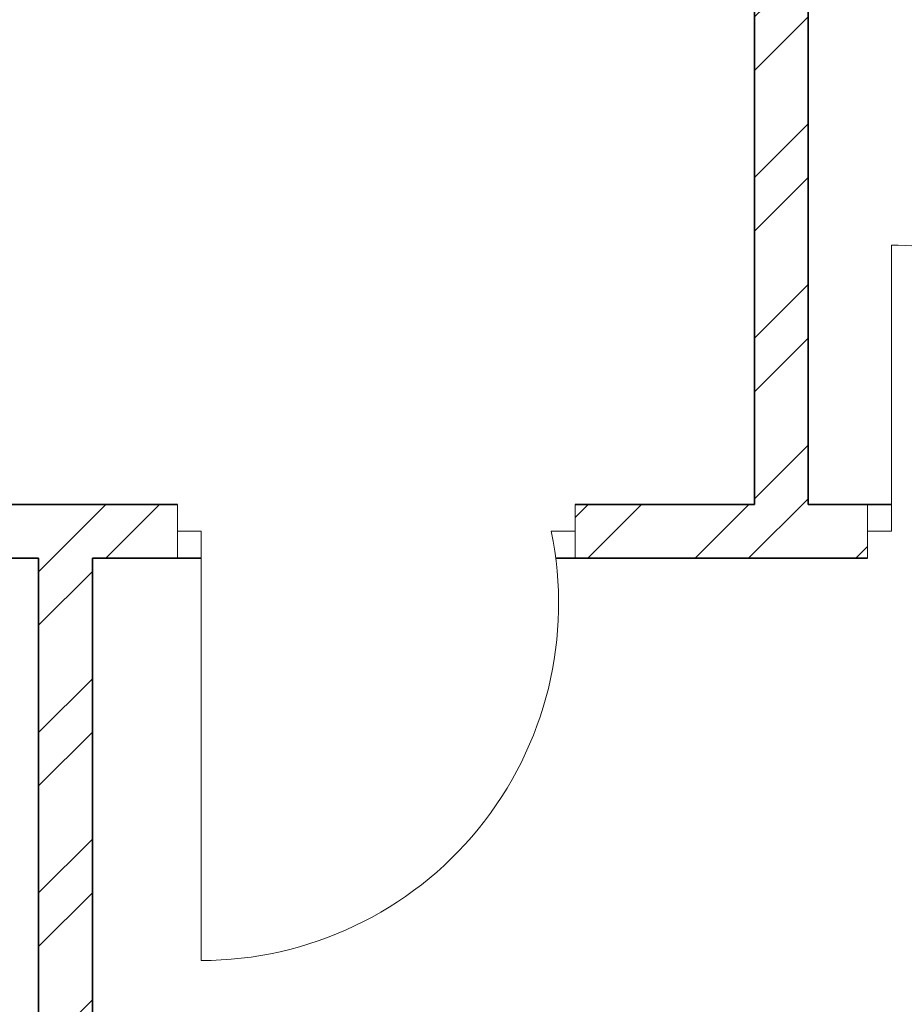
# Model space of a CAD drawing. Units: inches. Extents: x 1962 to 2771, y 1245 to 2660.
# Tile 14 of 114: x 2506 to 2580, y 1609 to 1692. Entities that reach past the tile are written whole.
import ezdxf

# ---------------------------------------------------------------- set-up
doc = ezdxf.new("R2010")
doc.units = ezdxf.units.IN
for name, color, linetype, lineweight in [('A-DOOR', 3, 'Continuous', 18), ('A-WALL', 7, 'Continuous', 35), ('A-WALL-PATT', 252, 'Continuous', 13)]:
    doc.layers.add(name, color=color, linetype=linetype, lineweight=lineweight)

msp = doc.modelspace()

# ---------------------------------------------------------------- hatches: boundary and pattern name
at = {"layer": 'A-WALL-PATT'}
h = msp.add_hatch(dxfattribs=at)
h.set_pattern_fill('ANSI32', color=256)
h.paths.add_polyline_path([(2090.8074, 2467.3437), (2141.6481, 2467.3437), (2141.6481, 2469.5937), (2141.6481, 2471.8437), (2086.3074, 2471.8437), (2086.3074, 2422.5333), (2090.8074, 2422.5333)])
h.paths.add_polyline_path([(2282.7664, 2471.8437), (2204.8982, 2471.8437), (2204.8982, 2467.3437), (2234.8074, 2467.3437), (2234.8074, 2311.3437), (2228.7492, 2311.3437), (2228.7492, 2306.8437), (2234.8074, 2306.8437), (2331.9227, 2306.8437), (2331.9227, 2309.0937), (2331.9227, 2311.3437), (2239.3074, 2311.3437), (2239.3074, 2467.3437), (2282.7664, 2467.3437), (2282.7664, 2469.5937)])
h.paths.add_polyline_path([(2471.4531, 2519.8437), (2552.011, 2519.8437), (2564.3996, 2519.8437), (2564.3996, 2511.1389), (2568.8996, 2511.1389), (2568.8996, 2524.3437), (2466.9531, 2524.3437), (2466.9531, 2471.8437), (2450.0749, 2471.8437), (2446.4672, 2471.8437), (2446.4672, 2467.3437), (2450.0749, 2467.3437), (2475.9988, 2467.3437), (2475.9988, 2469.5937), (2475.9988, 2471.8437), (2471.4531, 2471.8437)])
h.paths.add_polyline_path([(2575.2231, 2469.5937), (2575.2231, 2471.8437), (2568.8996, 2471.8437), (2568.8996, 2487.1389), (2564.3996, 2487.1389), (2564.3996, 2471.8437), (2556.511, 2471.8437), (2499.2904, 2471.8437), (2499.2904, 2467.3437), (2507.8074, 2467.3437), (2507.8074, 2311.3437), (2414.863, 2311.3437), (2414.863, 2306.8437), (2512.3074, 2306.8437), (2517.0114, 2306.8437), (2517.0114, 2309.0937), (2517.0114, 2311.3437), (2512.3074, 2311.3437), (2512.3074, 2467.3437), (2575.2231, 2467.3437)])
h.paths.add_polyline_path([(2660.8074, 2471.8437), (2600.9602, 2471.8437), (2600.9602, 2467.3437), (2656.3074, 2467.3437), (2656.3074, 2432.5704), (2660.8074, 2432.5704)])
h.paths.add_polyline_path([(2660.8074, 2372.5704), (2656.3074, 2372.5704), (2656.3074, 2311.3437), (2600.276, 2311.3437), (2600.276, 2309.0937), (2600.276, 2306.8437), (2656.3074, 2306.8437), (2656.3074, 2296.2593), (2660.8074, 2296.2593)])
h.paths.add_polyline_path([(2572.3074, 2306.8437), (2577.1385, 2306.8437), (2577.1385, 2311.3437), (2551.082, 2311.3437), (2551.082, 2306.8437), (2567.8074, 2306.8437), (2567.8074, 2258.8437), (2540.0574, 2258.8437), (2540.0574, 2256.5937), (2540.0574, 2254.3437), (2567.8074, 2254.3437), (2656.3074, 2254.3437), (2656.3074, 2236.9085), (2660.8074, 2236.9085), (2660.8074, 2272.2593), (2656.3074, 2272.2593), (2656.3074, 2258.8437), (2572.3074, 2258.8437)])
h.paths.add_polyline_path([(2512.3074, 2254.3437), (2518.8716, 2254.3437), (2518.8716, 2256.5937), (2518.8716, 2258.8437), (2507.8074, 2258.8437), (2507.8074, 2177.8437), (2567.8074, 2177.8437), (2567.8074, 2172.9628), (2572.3074, 2172.9628), (2572.3074, 2177.8437), (2656.3074, 2177.8437), (2656.3074, 2166.4846), (2660.8074, 2166.4846), (2660.8074, 2200.9085), (2656.3074, 2200.9085), (2656.3074, 2182.3437), (2512.3074, 2182.3437)])
h.paths.add_polyline_path([(2656.3074, 2129.8437), (2572.3074, 2129.8437), (2572.3074, 2150.3044), (2570.0574, 2150.3044), (2567.8074, 2150.3044), (2567.8074, 2129.8437), (2507.8074, 2129.8437), (2507.8074, 2116.3027), (2510.0574, 2116.3027), (2512.3074, 2116.3027), (2512.3074, 2125.3437), (2567.8074, 2125.3437), (2572.3074, 2125.3437), (2656.3074, 2125.3437)])
h.paths.add_polyline_path([(2090.8074, 2362.5333), (2086.3074, 2362.5333), (2086.3074, 2298.6242), (2090.8074, 2298.6242), (2090.8074, 2306.8437), (2174.8074, 2306.8437), (2174.8074, 2286.4178), (2179.3074, 2286.4178), (2179.3074, 2306.8437), (2192.8641, 2306.8437), (2192.8641, 2309.0937), (2192.8641, 2311.3437), (2090.8074, 2311.3437)])
h.paths.add_polyline_path([(2209.156, 2258.8437), (2179.3074, 2258.8437), (2179.3074, 2263.2236), (2177.0574, 2263.2236), (2174.8074, 2263.2236), (2174.8074, 2258.8437), (2090.8074, 2258.8437), (2090.8074, 2274.6242), (2086.3074, 2274.6242), (2086.3074, 2238.2967), (2088.5574, 2238.2967), (2090.8074, 2238.2967), (2090.8074, 2254.3437), (2209.156, 2254.3437)])
h.paths.add_polyline_path([(2090.8074, 2177.8437), (2234.8074, 2177.8437), (2234.8074, 2173.1428), (2239.3074, 2173.1428), (2239.3074, 2258.8437), (2230.8442, 2258.8437), (2230.8442, 2256.5937), (2230.8442, 2254.3437), (2234.8074, 2254.3437), (2234.8074, 2182.3437), (2090.8074, 2182.3437), (2090.8074, 2202.2967), (2086.3074, 2202.2967), (2086.3074, 2140.0389), (2090.8074, 2140.0389)])
h.paths.add_polyline_path([(2090.8074, 2080.0389), (2086.3074, 2080.0389), (2086.3074, 2033.8437), (2090.8074, 2033.8437)], flags=17)
h.paths.add_polyline_path([(2244.9405, 2033.8437), (2239.3074, 2033.8437), (2239.3074, 2142.0665), (2237.2592, 2142.0665), (2234.8074, 2142.0665), (2234.8074, 2033.8437), (2090.8074, 2033.8437), (2076.5204, 2033.8437), (2072.0204, 2033.8437), (2072.0204, 2000.4493), (2076.5204, 2000.4493), (2076.5204, 2029.3437), (2090.8074, 2029.3437), (2244.9405, 2029.3437), (2244.9405, 2031.5937)])
h.paths.add_polyline_path([(2234.8074, 1933.3437), (2076.5204, 1933.3437), (2076.5204, 1952.4493), (2074.2704, 1952.4493), (2072.0204, 1952.4493), (2072.0204, 1933.3437), (2072.0204, 1928.8437), (2234.8074, 1928.8437)])
h.paths.add_polyline_path([(2090.8074, 1928.8437), (2086.3074, 1928.8437), (2086.3074, 1906.5013), (2090.8074, 1906.5013)])
h.paths.add_polyline_path([(2090.8074, 1846.5013), (2086.3074, 1846.5013), (2086.3074, 1769.9917), (2088.5574, 1769.9917), (2090.8074, 1769.9917), (2090.8074, 1780.3437), (2234.8074, 1780.3437), (2234.8074, 1708.3437), (2230.3764, 1708.3437), (2230.3764, 1703.8437), (2239.3074, 1703.8437), (2239.3074, 1792.6669), (2237.0574, 1792.6669), (2234.8074, 1792.6669), (2234.8074, 1784.8437), (2090.8074, 1784.8437)])
h.paths.add_polyline_path([(2239.3074, 1928.8437), (2244.9405, 1928.8437), (2244.9405, 1931.0937), (2244.9405, 1933.3437), (2234.8074, 1933.3437), (2234.8074, 1928.8437), (2234.8074, 1825.5949), (2239.3074, 1825.5949)])
h.paths.add_polyline_path([(2148.0425, 1649.0937), (2148.0425, 1651.3437), (2090.8074, 1651.3437), (2090.8074, 1646.8437), (2148.0425, 1646.8437)], flags=0)
h.paths.add_polyline_path([(2207.5601, 1708.3437), (2090.8074, 1708.3437), (2090.8074, 1703.8437), (2174.8074, 1703.8437), (2174.8074, 1651.3437), (2170.4457, 1651.3437), (2170.4457, 1646.8437), (2195.9924, 1646.8437), (2195.9924, 1649.0937), (2195.9924, 1651.3437), (2179.3074, 1651.3437), (2179.3074, 1703.8437), (2207.5601, 1703.8437), (2207.5601, 1706.0937)])
h.paths.add_polyline_path([(2090.8074, 1733.9917), (2086.3074, 1733.9917), (2086.3074, 1696.1032), (2088.5574, 1696.1032), (2090.8074, 1696.1032)])
h.paths.add_polyline_path([(2090.8074, 1672.1032), (2086.3074, 1672.1032), (2086.3074, 1600.3335), (2090.8074, 1600.3335)])
h.paths.add_polyline_path([(2090.8074, 1540.3335), (2086.3074, 1540.3335), (2086.3074, 1486.3437), (2139.6766, 1486.3437), (2139.6766, 1490.8437), (2090.8074, 1490.8437)])
h.paths.add_polyline_path([(2302.3876, 1490.8437), (2239.3074, 1490.8437), (2239.3074, 1646.8437), (2335.9994, 1646.8437), (2335.9994, 1651.3437), (2229.884, 1651.3437), (2229.884, 1646.8437), (2234.8074, 1646.8437), (2234.8074, 1490.8437), (2202.7103, 1490.8437), (2202.7103, 1488.5937), (2202.7103, 1486.3437), (2275.0699, 1486.3437), (2275.0699, 1475.772), (2279.5699, 1475.772), (2279.5699, 1486.3437), (2302.3876, 1486.3437)])
h.paths.add_polyline_path([(2279.5699, 1451.772), (2275.0699, 1451.772), (2275.0699, 1438.3437), (2174.8074, 1438.3437), (2174.8074, 1486.3437), (2179.7922, 1486.3437), (2179.7922, 1490.8437), (2163.3585, 1490.8437), (2163.3585, 1488.5937), (2163.3585, 1486.3437), (2170.3074, 1486.3437), (2170.3074, 1433.8437), (2279.5699, 1433.8437)])
h.paths.add_polyline_path([(2427.2363, 1490.8437), (2375.8074, 1490.8437), (2375.8074, 1646.8437), (2381.6401, 1646.8437), (2381.6401, 1651.3437), (2365.887, 1651.3437), (2365.887, 1649.0937), (2365.887, 1646.8437), (2371.3074, 1646.8437), (2371.3074, 1490.8437), (2327.5627, 1490.8437), (2327.5627, 1488.5937), (2327.5627, 1486.3437), (2371.3074, 1486.3437), (2371.3074, 1433.8437), (2375.8074, 1433.8437), (2375.8074, 1486.3437), (2427.2363, 1486.3437)])
h.paths.add_polyline_path([(2512.3074, 1646.8437), (2519.4351, 1646.8437), (2519.4351, 1649.0937), (2519.4351, 1651.3437), (2507.8074, 1651.3437), (2416.0063, 1651.3437), (2416.0063, 1649.0937), (2416.0063, 1646.8437), (2507.8074, 1646.8437), (2507.8074, 1490.8437), (2497.0532, 1490.8437), (2497.0532, 1488.5937), (2497.0532, 1486.3437), (2574.9344, 1486.3437), (2574.9344, 1476.0181), (2579.4344, 1476.0181), (2579.4344, 1486.3437), (2584.4872, 1486.3437), (2584.3074, 1490.8437), (2512.3074, 1490.8437)])
h.paths.add_polyline_path([(2470.5091, 1486.3437), (2473.9767, 1486.3437), (2473.9767, 1490.8437), (2449.6605, 1490.8437), (2449.6605, 1488.5937), (2449.6605, 1486.3437), (2466.0091, 1486.3437), (2466.0091, 1433.8437), (2470.5091, 1433.8437), (2579.4344, 1433.8437), (2579.4344, 1452.0181), (2574.9344, 1452.0181), (2574.9344, 1438.3437), (2554.5091, 1438.3437), (2470.5091, 1438.3437)])
h.paths.add_polyline_path([(2656.3074, 1490.8437), (2611.86, 1490.8437), (2611.86, 1486.3437), (2656.3074, 1486.3437)])
h.paths.add_polyline_path([(2660.8074, 1532.7007), (2658.5574, 1532.7007), (2656.3074, 1532.7007), (2656.3074, 1486.3437), (2660.8074, 1486.3437)])
h.paths.add_polyline_path([(2660.8074, 1664.9663), (2656.3074, 1664.9663), (2656.3074, 1651.3437), (2602.2313, 1651.3437), (2602.2313, 1646.8437), (2656.3074, 1646.8437), (2656.3074, 1592.7007), (2660.8074, 1592.7007)])
h.paths.add_polyline_path([(2660.8074, 1724.5221), (2656.3074, 1724.5221), (2656.3074, 1703.8437), (2542.4725, 1703.8437), (2542.4725, 1699.3437), (2567.8074, 1699.3437), (2567.8074, 1651.3437), (2552.7766, 1651.3437), (2552.7766, 1649.0937), (2552.7766, 1646.8437), (2577.2878, 1646.8437), (2577.2878, 1649.0937), (2577.2878, 1651.3437), (2572.3074, 1651.3437), (2572.3074, 1699.3437), (2656.3074, 1699.3437), (2656.3074, 1688.9663), (2660.8074, 1688.9663)])
h.paths.add_polyline_path([(2660.8074, 1880.6524), (2656.3074, 1880.6524), (2656.3074, 1832.8437), (2512.3074, 1832.8437), (2512.3074, 1837.8959), (2507.8074, 1837.8959), (2507.8074, 1828.3437), (2567.8074, 1828.3437), (2567.8074, 1804.3437), (2572.3074, 1804.3437), (2572.3074, 1828.3437), (2656.3074, 1828.3437), (2656.3074, 1818.6778), (2660.8074, 1818.6778)])
h.paths.add_polyline_path([(2660.8074, 1794.6778), (2656.3074, 1794.6778), (2656.3074, 1780.3437), (2572.3074, 1780.3437), (2572.3074, 1783.0303), (2570.0574, 1783.0303), (2567.8074, 1783.0303), (2567.8074, 1780.3437), (2507.8074, 1780.3437), (2507.8074, 1699.3437), (2517.8858, 1699.3437), (2517.8858, 1701.5937), (2517.8858, 1703.8437), (2512.3074, 1703.8437), (2512.3074, 1775.8437), (2656.3074, 1775.8437), (2656.3074, 1760.5221), (2660.8074, 1760.5221)])
h.paths.add_polyline_path([(2660.8074, 1981.3437), (2660.8074, 2020.2808), (2658.5574, 2020.2808), (2656.3074, 2020.2808), (2656.3074, 1981.3437), (2512.3074, 1981.3437), (2512.3074, 2086.6996), (2507.8074, 2086.6996), (2507.8074, 1981.3437), (2375.8074, 1981.3437), (2375.8074, 1986.8505), (2373.5574, 1986.8505), (2371.3074, 1986.8505), (2371.3074, 1973.2607), (2375.8074, 1973.2607), (2375.8074, 1976.8437), (2507.8074, 1976.8437), (2507.8074, 1865.4281), (2510.0574, 1865.4281), (2512.3074, 1865.4281), (2512.3074, 1976.8437), (2660.8074, 1976.8437)])
h.paths.add_polyline_path([(2375.8074, 1940.297), (2373.5574, 1940.297), (2371.3074, 1940.297), (2371.3074, 1933.3437), (2278.4434, 1933.3437), (2278.4434, 1928.8437), (2371.3074, 1928.8437), (2371.3074, 1651.3437), (2375.8074, 1651.3437)])
h.paths.add_polyline_path([(2660.8074, 1976.8437), (2656.3074, 1976.8437), (2656.3074, 1940.6524), (2660.8074, 1940.6524)], flags=17)
h.paths.add_polyline_path([(2660.8074, 2142.4846), (2656.3074, 2142.4846), (2656.3074, 2080.2808), (2660.8074, 2080.2808)])
h.paths.add_polyline_path([(2381.4189, 2311.3437), (2375.8074, 2311.3437), (2375.8074, 2467.3437), (2424.7242, 2467.3437), (2424.7242, 2469.5937), (2424.7242, 2471.8437), (2375.8074, 2471.8437), (2375.8074, 2524.3437), (2371.3074, 2524.3437), (2371.3074, 2471.8437), (2307.2097, 2471.8437), (2307.2097, 2467.3437), (2371.3074, 2467.3437), (2371.3074, 2311.3437), (2366.8901, 2311.3437), (2366.8901, 2306.8437), (2371.3074, 2306.8437), (2371.3074, 2033.8437), (2279.6589, 2033.8437), (2279.6589, 2029.3437), (2371.3074, 2029.3437), (2371.3074, 2014.2598), (2375.8074, 2014.2598), (2375.8074, 2306.8437), (2381.4189, 2306.8437)])
h.paths.add_polyline_path([(2263.3074, 2524.3437), (2170.3074, 2524.3437), (2170.3074, 2519.8437), (2170.3074, 2471.8437), (2165.0312, 2471.8437), (2165.0312, 2467.3437), (2179.6721, 2467.3437), (2179.6721, 2469.5161), (2179.6721, 2471.8437), (2174.8074, 2471.8437), (2174.8074, 2519.8437), (2258.8074, 2519.8437), (2258.8074, 2511.6436), (2263.3074, 2511.6436)])
h.paths.add_polyline_path([(2245.0232, 1361.4123), (2492.9468, 1361.4123), (2492.9468, 1398.505), (2245.0232, 1398.505)], flags=9)
h.paths.add_polyline_path([(2388.1434, 2086.6936), (2425.0704, 2086.6936), (2425.0704, 2105.3509), (2388.1434, 2105.3509)], flags=9)
h.paths.add_polyline_path([(2404.922, 2242.6744), (2445.7337, 2242.6744), (2445.7337, 2261.3318), (2404.922, 2261.3318)], flags=9)
h.paths.add_polyline_path([(2269.4107, 2156.7935), (2306.3378, 2156.7935), (2306.3378, 2175.4508), (2269.4107, 2175.4508)], flags=9)
h.paths.add_polyline_path([(2269.3277, 2233.4343), (2306.2547, 2233.4343), (2306.2547, 2252.0917), (2269.3277, 2252.0917)], flags=9)
h.paths.add_polyline_path([(2431.6052, 2320.6922), (2470.4456, 2320.6922), (2470.4456, 2339.3495), (2431.6052, 2339.3495)], flags=25)
h.paths.add_polyline_path([(2249.6902, 2315.7608), (2288.5306, 2315.7608), (2288.5306, 2334.4182), (2249.6902, 2334.4182)], flags=25)
h.paths.add_polyline_path([(2096.9301, 2314.3181), (2135.7704, 2314.3181), (2135.7704, 2332.9755), (2096.9301, 2332.9755)], flags=25)
h.paths.add_polyline_path([(2134.3475, 2285.7089), (2161.4655, 2285.7089), (2161.4655, 2304.3662), (2134.3475, 2304.3662)], flags=9)
h.paths.add_polyline_path([(2126.5155, 2209.4076), (2159.9227, 2209.4076), (2159.9227, 2228.065), (2126.5155, 2228.065)], flags=25)
h.paths.add_polyline_path([(2110.5753, 2141.5299), (2149.4157, 2141.5299), (2149.4157, 2160.1872), (2110.5753, 2160.1872)], flags=25)
h.paths.add_polyline_path([(2249.8618, 1968.3317), (2286.3966, 1968.3317), (2286.3966, 1986.989), (2249.8618, 1986.989)], flags=9)
h.paths.add_polyline_path([(2395.9507, 1777.0051), (2436.7624, 1777.0051), (2436.7624, 1795.6625), (2395.9507, 1795.6625)], flags=9)
h.paths.add_polyline_path([(2398.5259, 1888.5651), (2435.0062, 1888.5651), (2435.0062, 1907.2224), (2398.5259, 1907.2224)], flags=25)
h.paths.add_polyline_path([(2259.3506, 1728.3559), (2296.2776, 1728.3559), (2296.2776, 1747.0132), (2259.3506, 1747.0132)], flags=9)
h.paths.add_polyline_path([(2271.3698, 1845.268), (2308.2968, 1845.268), (2308.2968, 1863.9253), (2271.3698, 1863.9253)], flags=9)
h.paths.add_polyline_path([(2120.9355, 1786.3027), (2159.7759, 1786.3027), (2159.7759, 1804.9601), (2120.9355, 1804.9601)], flags=25)
h.paths.add_polyline_path([(2121.3164, 1732.1043), (2154.7236, 1732.1043), (2154.7236, 1750.7616), (2121.3164, 1750.7616)], flags=25)
h.paths.add_polyline_path([(2118.3706, 1678.8997), (2147.5282, 1678.8997), (2147.5282, 1697.557), (2118.3706, 1697.557)], flags=25)
h.paths.add_polyline_path([(2385.9227, 1493.557), (2424.763, 1493.557), (2424.763, 1512.2143), (2385.9227, 1512.2143)], flags=25)
h.paths.add_polyline_path([(2248.7058, 1500.0256), (2287.5462, 1500.0256), (2287.5462, 1518.6829), (2248.7058, 1518.6829)], flags=25)
h.paths.add_polyline_path([(2104.1669, 1617.3771), (2143.0073, 1617.3771), (2143.0073, 1636.0344), (2104.1669, 1636.0344)], flags=9)
h.paths.add_polyline_path([(2096.0714, 1447.8824), (2137.3845, 1447.8824), (2137.3845, 1458.1859), (2096.0714, 1458.1859)], flags=9)
h.paths.add_polyline_path([(2180.6114, 1440.325), (2209.7689, 1440.325), (2209.7689, 1458.9823), (2180.6114, 1458.9823)], flags=25)
h.paths.add_polyline_path([(2316.1698, 1447.9637), (2357.4829, 1447.9637), (2357.4829, 1458.2673), (2316.1698, 1458.2673)], flags=9)
h.paths.add_polyline_path([(2397.6187, 1447.9637), (2438.9318, 1447.9637), (2438.9318, 1458.2673), (2397.6187, 1458.2673)], flags=9)
h.paths.add_polyline_path([(2473.0778, 1439.5953), (2502.2354, 1439.5953), (2502.2354, 1458.2527), (2473.0778, 1458.2527)], flags=25)
h.paths.add_polyline_path([(2589.7027, 1447.8819), (2631.0158, 1447.8819), (2631.0158, 1458.1855), (2589.7027, 1458.1855)], flags=9)
h.paths.add_polyline_path([(2522.4009, 1497.5285), (2561.2413, 1497.5285), (2561.2413, 1516.1859), (2522.4009, 1516.1859)], flags=25)
h.paths.add_polyline_path([(2579.6565, 1671.3482), (2608.8141, 1671.3482), (2608.8141, 1690.0056), (2579.6565, 1690.0056)], flags=25)
h.paths.add_polyline_path([(2544.7038, 1725.5064), (2578.1111, 1725.5064), (2578.1111, 1744.1637), (2544.7038, 1744.1637)], flags=25)
h.paths.add_polyline_path([(2578.1191, 1807.472), (2607.2766, 1807.472), (2607.2766, 1826.1293), (2578.1191, 1826.1293)], flags=25)
h.paths.add_polyline_path([(2595.0614, 1835.1839), (2633.9018, 1835.1839), (2633.9018, 1853.8413), (2595.0614, 1853.8413)], flags=25)
h.paths.add_polyline_path([(2567.0097, 2097.7035), (2605.8501, 2097.7035), (2605.8501, 2116.3609), (2567.0097, 2116.3609)], flags=9)
h.paths.add_polyline_path([(2586.644, 2134.6454), (2615.8015, 2134.6454), (2615.8015, 2153.3027), (2586.644, 2153.3027)], flags=9)
h.paths.add_polyline_path([(2544.6185, 2212.6783), (2578.0258, 2212.6783), (2578.0258, 2231.3356), (2544.6185, 2231.3356)], flags=25)
h.paths.add_polyline_path([(2577.0273, 2256.9023), (2606.1849, 2256.9023), (2606.1849, 2275.5597), (2577.0273, 2275.5597)], flags=24)
h.paths.add_polyline_path([(2605.2683, 2315.2821), (2644.1087, 2315.2821), (2644.1087, 2333.9395), (2605.2683, 2333.9395)], flags=25)
h.paths.add_polyline_path([(2583.1244, 2496.1815), (2624.4375, 2496.1815), (2624.4375, 2506.4851), (2583.1244, 2506.4851)], flags=9)
h.paths.add_polyline_path([(2474.761, 2497.0823), (2503.9185, 2497.0823), (2503.9185, 2515.7397), (2474.761, 2515.7397)], flags=25)
h.paths.add_polyline_path([(2387.5787, 2494.2563), (2428.902, 2494.2563), (2428.902, 2504.5598), (2387.5787, 2504.5598)], flags=9)
h.paths.add_polyline_path([(2300.1657, 2500.1564), (2341.4788, 2500.1564), (2341.4788, 2510.46), (2300.1657, 2510.46)], flags=25)
h.paths.add_polyline_path([(2176.8589, 2497.5843), (2206.0165, 2497.5843), (2206.0165, 2516.2416), (2176.8589, 2516.2416)], flags=25)
h.paths.add_polyline_path([(2097.4668, 2494.9762), (2138.7799, 2494.9762), (2138.7799, 2505.2798), (2097.4668, 2505.2798)], flags=9)

# ---------------------------------------------------------------- linework, layer by layer
at = {"layer": 'A-DOOR'}
for p, q in [((2579.2878, 1649.0937), (2579.2878, 1673.0937)), ((2519.4351, 1651.3437), (2519.4351, 1646.8437)), ((2552.7766, 1646.8437), (2552.7766, 1651.3437)), ((2552.7766, 1651.3437), (2552.7766, 1649.0937)), ((2577.2878, 1651.3437), (2577.2878, 1646.8437)), ((2519.4351, 1646.8437), (2519.4351, 1649.0937)), ((2519.4351, 1649.0937), (2521.4351, 1649.0937)), ((2521.4351, 1649.0937), (2521.4351, 1613.0937)), ((2552.7766, 1649.0937), (2550.7766, 1649.0937)), ((2577.2878, 1646.8437), (2577.2878, 1649.0937)), ((2577.2878, 1649.0937), (2579.2878, 1649.0937))]:
    msp.add_line(p, q, dxfattribs=at)
for centre, radius, start, end in [((2579.2878, 1651.9556), 21.1381, 352.218733, 90), ((2521.4351, 1643.051), 29.9573, 270, 11.63702)]:
    msp.add_arc(centre, radius, start, end, dxfattribs=at)
at = {"layer": 'A-WALL'}
for p, q in [((2567.8074, 1651.3437), (2567.8074, 1699.3437)), ((2572.3074, 1699.3437), (2572.3074, 1651.3437)), ((2507.8074, 1651.3437), (2416.0063, 1651.3437)), ((2519.4351, 1651.3437), (2507.8074, 1651.3437)), ((2567.8074, 1651.3437), (2552.7766, 1651.3437)), ((2579.2878, 1651.3437), (2572.3074, 1651.3437)), ((2507.8074, 1646.8437), (2414.3062, 1646.8437)), ((2507.8074, 1646.8437), (2507.8074, 1490.8437)), ((2512.3074, 1646.8437), (2512.3074, 1490.8437)), ((2521.4351, 1646.8437), (2512.3074, 1646.8437)), ((2577.2878, 1646.8437), (2551.1513, 1646.8437)), ((2572.3074, 1646.8437), (2567.8074, 1646.8437))]:
    msp.add_line(p, q, dxfattribs=at)

doc.saveas('drawing.dxf')
